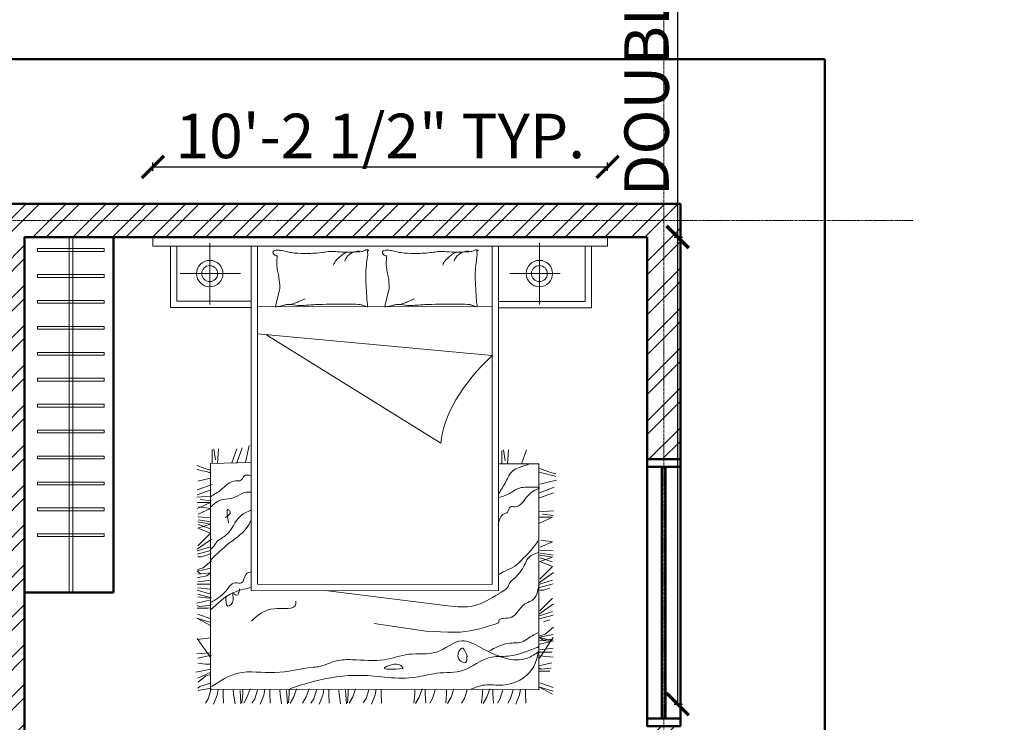
# Model space of a CAD drawing. Units: inches. Extents: x 261 to 2725, y 291 to 1454.
# Tile 15 of 35: x 777 to 1043, y 1091 to 1281. Entities that reach past the tile are written whole.
import ezdxf

# ---------------------------------------------------------------- set-up
doc = ezdxf.new("R2010")
doc.units = ezdxf.units.IN
doc.linetypes.add('CENTER', pattern=[2, 1.25, -0.25, 0.25, -0.25])
for name, color, linetype, lineweight in [('A-ANNO-DIMS', 136, 'Continuous', 18), ('A-FURN', 30, 'Continuous', 18), ('A-GRID', 251, 'CENTER', 13), ('A-WALL', 222, 'Continuous', 50), ('A-WALL-PATT', 243, 'Continuous', 13)]:
    doc.layers.add(name, color=color, linetype=linetype, lineweight=lineweight)
doc.styles.get("Standard").update_dxf_attribs({"font": 'arial.ttf'})
doc.dimstyles.new('ISO-25', dxfattribs={"dimtxt": 12, "dimasz": 6, "dimexe": 1.25, "dimexo": 0.625, "dimtad": 1, "dimdec": 0, "dimlunit": 3, "dimtxsty": 'Standard', "dimblk": 'ARCHTICK', "dimcen": 2.5, "dimadec": 0, "dimazin": 0, "dimtfac": 1, "dimtdec": 0, "dimtmove": 0, "dimatfit": 3, "dimfxl": 1, "dimfxlon": 1, "dimarcsym": 0})

# ---------------------------------------------------------------- blocks, each defined once
blk = doc.blocks.new('A$C2B723114')
for p, q in [((0, 2.9047), (2.8274, 2.9047)), ((0, 2.8487), (0, 2.9047)), ((2.8274, 2.9047), (2.8274, 2.8487)), ((2.8274, 2.8487), (0, 2.8487)), ((0.1012, 2.4649), (0.1012, 2.849)), ((0.1396, 2.5033), (0.1396, 2.849)), ((0.4243, 2.8697), (0.4243, 2.4855)), ((0.6794, 0.7051), (0.6794, 2.8509)), ((0.7187, 0.7435), (0.7187, 2.8509)), ((2.1776, 2.8509), (2.1776, 0.7454)), ((2.216, 2.8509), (2.216, 0.707)), ((2.4742, 2.8697), (2.4742, 2.4855)), ((2.6798, 2.5052), (2.6798, 2.8509)), ((2.7182, 2.4668), (2.7182, 2.8509)), ((0.6087, 2.6776), (0.295, 2.6776)), ((2.6586, 2.6776), (2.2821, 2.6776)), ((1.3789, 2.4999), (1.3598, 2.5761)), ((2.0593, 2.4999), (2.0402, 2.5761)), ((0.6794, 2.4649), (0.1012, 2.4649)), ((0.6766, 2.5033), (0.1396, 2.5033)), ((0.7191, 2.47), (2.1778, 2.4719)), ((1.3858, 2.4723), (1.3789, 2.4999)), ((2.0662, 2.4723), (2.0593, 2.4999)), ((2.2188, 2.5052), (2.6798, 2.5052)), ((2.2188, 2.4668), (2.7182, 2.4668)), ((2.1771, 2.3036), (0.718, 2.1685)), ((1.0365, 1.6233), (2.1246, 2.2989)), ((2.2287, 1.6076), (2.2523, 1.5035)), ((2.2726, 1.593), (2.3061, 1.5007)), ((0.5047, 1.5819), (0.5353, 1.4945)), ((0.6174, 1.5819), (0.6232, 1.4916)), ((0.6467, 1.5819), (0.6369, 1.5137)), ((0.6571, 1.4945), (0.6571, 1.5765)), ((2.3067, 1.5881), (2.3373, 1.5007)), ((2.4194, 1.5881), (2.4251, 1.4979)), ((2.4487, 1.5881), (2.4389, 1.5199)), ((2.4591, 1.5007), (2.4591, 1.5828)), ((0.4269, 0.0884), (0.4269, 1.4945)), ((0.4269, 1.4945), (0.6794, 1.4945)), ((2.4685, 1.4964), (2.216, 1.5022)), ((2.4685, 1.4964), (2.4685, 0.0903)), ((0.3172, 1.3923), (0.4213, 1.3687)), ((0.3318, 1.3485), (0.4241, 1.3149)), ((2.4596, 1.3659), (2.552, 1.3324)), ((2.4685, 1.4044), (2.5491, 1.3861)), ((0.3367, 1.3143), (0.4241, 1.2838)), ((2.4645, 1.3318), (2.552, 1.3012)), ((2.4645, 1.2928), (2.5548, 1.2871)), ((2.4645, 1.2635), (2.5328, 1.2733)), ((2.4699, 1.2531), (2.552, 1.2163)), ((2.552, 1.2531), (2.4699, 1.2531)), ((2.5435, 1.2276), (2.4699, 1.2163)), ((0.3367, 1.2016), (0.427, 1.1959)), ((0.3367, 1.1724), (0.405, 1.1821)), ((2.5491, 1.1654), (2.467, 1.1597)), ((2.4699, 1.2163), (2.5463, 1.1823)), ((0.4241, 1.162), (0.3421, 1.162)), ((0.3421, 1.162), (0.4241, 1.1252)), ((2.5463, 1.1455), (2.467, 1.1342)), ((2.5491, 1.1342), (2.4699, 1.1201)), ((2.4699, 1.1201), (2.5491, 1.0946)), ((2.5463, 1.1172), (2.4727, 1.0918)), ((2.5491, 1.0946), (2.4699, 1.0635)), ((2.4699, 1.0635), (2.5491, 0.9842)), ((0.4157, 1.0206), (0.3421, 1.0093)), ((0.3421, 1.0093), (0.4185, 0.9754)), ((2.4642, 1.0267), (2.552, 0.9644)), ((0.4213, 0.9584), (0.3392, 0.9527)), ((0.4185, 0.9386), (0.3392, 0.9272)), ((0.4213, 0.9272), (0.3421, 0.9131)), ((2.4642, 0.9389), (2.4869, 0.9276)), ((2.467, 0.9559), (2.552, 0.9333)), ((2.4699, 0.9785), (2.552, 0.9531)), ((2.4869, 0.9276), (2.5265, 0.9163)), ((0.3421, 0.9131), (0.4213, 0.8876)), ((0.4213, 0.8876), (0.3421, 0.8565)), ((0.4185, 0.9103), (0.3449, 0.8848)), ((2.4642, 0.8908), (2.5152, 0.8483)), ((2.5265, 0.9163), (2.5491, 0.9163)), ((0.3364, 0.8197), (0.4241, 0.7574)), ((0.3421, 0.8565), (0.4213, 0.7772)), ((2.467, 0.8455), (2.5208, 0.8342)), ((2.4699, 0.8172), (2.4925, 0.7974)), ((2.5491, 0.8087), (2.4699, 0.8172)), ((2.4925, 0.7974), (2.535, 0.7889)), ((2.5152, 0.8483), (2.5491, 0.837)), ((2.5208, 0.8342), (2.552, 0.8285)), ((2.552, 0.8285), (2.5293, 0.8087)), ((0.3392, 0.7489), (0.4241, 0.7263)), ((0.3421, 0.7716), (0.4241, 0.7461)), ((2.1776, 0.7454), (0.7187, 0.7435)), ((2.5491, 0.7606), (2.467, 0.7719)), ((2.4727, 0.7464), (2.467, 0.7408)), ((2.552, 0.7464), (2.4727, 0.7464)), ((2.535, 0.7889), (2.552, 0.7861)), ((0.359, 0.7206), (0.3987, 0.7093)), ((0.3987, 0.7093), (0.4213, 0.7093)), ((2.216, 0.707), (0.6794, 0.7051)), ((0.9938, 0.6115), (1.7555, 0.7064)), ((2.5491, 0.6842), (2.4642, 0.6615)), ((2.467, 0.7153), (2.5491, 0.7238)), ((2.552, 0.7096), (2.467, 0.6842)), ((0.3364, 0.6233), (0.4241, 0.561)), ((0.3421, 0.6601), (0.4213, 0.5808)), ((2.4642, 0.6191), (2.4784, 0.6134)), ((2.5491, 0.6672), (2.4755, 0.6587)), ((2.4755, 0.6474), (2.5548, 0.6276)), ((2.4784, 0.6134), (2.5406, 0.6077)), ((2.5406, 0.6077), (2.552, 0.6134)), ((0.3392, 0.5525), (0.4241, 0.5299)), ((0.3421, 0.5752), (0.4241, 0.5497)), ((2.467, 0.5993), (2.4869, 0.5964)), ((2.467, 0.5313), (2.5491, 0.5596)), ((2.4869, 0.5964), (2.552, 0.5964)), ((0.359, 0.5242), (0.3987, 0.5129)), ((1.4523, 0.5021), (1.1305, 0.4537)), ((2.467, 0.5087), (2.5548, 0.5342)), ((2.5548, 0.5342), (2.4699, 0.4889)), ((0.3364, 0.4785), (0.3874, 0.436)), ((0.3392, 0.4332), (0.393, 0.4219)), ((0.3874, 0.436), (0.4213, 0.4247)), ((1.1305, 0.4537), (0.9938, 0.448)), ((0.4213, 0.415), (0.3364, 0.3923)), ((0.4241, 0.2868), (0.3392, 0.415)), ((0.3421, 0.4049), (0.3647, 0.3851)), ((0.4213, 0.3964), (0.3421, 0.4049)), ((0.4213, 0.398), (0.3477, 0.3895)), ((0.3647, 0.3851), (0.4072, 0.3766)), ((0.393, 0.4219), (0.4241, 0.4162)), ((0.4241, 0.4162), (0.4015, 0.3964)), ((0.4072, 0.3766), (0.4241, 0.3738)), ((2.467, 0.4133), (2.552, 0.4019)), ((2.467, 0.2879), (2.552, 0.4076)), ((0.4213, 0.3377), (0.3392, 0.3491)), ((0.4241, 0.3236), (0.3449, 0.3236)), ((2.467, 0.319), (2.5548, 0.3134)), ((0.3392, 0.2925), (0.4213, 0.3009)), ((0.3477, 0.2571), (0.427, 0.2373)), ((2.4642, 0.3049), (2.5491, 0.2851)), ((2.4699, 0.2491), (2.501, 0.2491)), ((2.501, 0.2491), (2.5491, 0.2547)), ((0.3506, 0.2231), (0.4128, 0.2175)), ((0.359, 0.2061), (0.4241, 0.2061)), ((0.4128, 0.2175), (0.4241, 0.2231)), ((2.467, 0.2179), (2.5605, 0.1981)), ((2.467, 0.1981), (2.5491, 0.1613)), ((2.467, 0.184), (2.4982, 0.1755)), ((0.3392, 0.1042), (0.4213, 0.1325)), ((2.4699, 0.1302), (2.535, 0.1104)), ((2.4982, 0.1755), (2.5463, 0.1359)), ((0.3392, 0.0815), (0.427, 0.107)), ((0.427, 0.107), (0.3421, 0.0617)), ((2.4685, 0.0903), (0.4269, 0.0884)), ((0.5106, 0.0657), (0.5077, 0.0063)), ((0.5106, 0.094), (0.5106, 0.0657)), ((0.5417, 0.094), (0.5474, 0.0572)), ((0.587, 0.0884), (0.604, 0.0346)), ((0.6512, 0.0884), (0.6682, 0.0346)), ((0.713, 0.0657), (0.7101, 0.0063)), ((0.713, 0.094), (0.713, 0.0657)), ((0.7334, 0.0943), (0.7503, 0.0434)), ((0.7786, 0.0915), (0.7786, 0.0632)), ((0.7786, 0.0632), (0.7843, 0.0066)), ((0.8739, 0.0884), (0.8908, 0.0346)), ((0.956, 0.0943), (0.973, 0.0434)), ((1.0013, 0.0915), (1.0013, 0.0632)), ((1.0013, 0.0632), (1.007, 0.0066)), ((1.072, 0.0884), (1.089, 0.0346)), ((1.1338, 0.0657), (1.131, 0.0063)), ((1.1338, 0.094), (1.1338, 0.0657)), ((1.1542, 0.0943), (1.1712, 0.0434)), ((1.1995, 0.0915), (1.1995, 0.0632)), ((1.1995, 0.0632), (1.2052, 0.0066)), ((1.4088, 0.0657), (1.406, 0.0063)), ((1.4088, 0.094), (1.4088, 0.0657)), ((1.44, 0.094), (1.4456, 0.0572)), ((1.4853, 0.0884), (1.5023, 0.0346)), ((1.5674, 0.0962), (1.5844, 0.0453)), ((1.6127, 0.0934), (1.6127, 0.0651)), ((1.6127, 0.0651), (1.6184, 0.0085)), ((1.6297, 0.0849), (1.624, 0.0028)), ((1.6693, 0.0623), (1.6608, 0.0028)), ((1.6721, 0.0877), (1.6693, 0.0623)), ((1.7344, 0.0651), (1.7316, 0.0057)), ((1.7344, 0.0934), (1.7344, 0.0651)), ((1.7655, 0.0934), (1.7712, 0.0566)), ((1.8108, 0.0877), (1.8278, 0.034)), ((1.8568, 0.0962), (1.8738, 0.0453)), ((1.9342, 0.0962), (1.9512, 0.0453)), ((1.9795, 0.0934), (1.9795, 0.0651)), ((1.9795, 0.0651), (1.9852, 0.0085)), ((1.9965, 0.0849), (1.9908, 0.0028)), ((2.0361, 0.0623), (2.0276, 0.0028)), ((2.039, 0.0877), (2.0361, 0.0623)), ((2.1012, 0.0651), (2.0984, 0.0057)), ((2.1012, 0.0934), (2.1012, 0.0651)), ((2.1324, 0.0934), (2.138, 0.0566)), ((2.1777, 0.0877), (2.1946, 0.034)), ((2.2236, 0.0962), (2.2406, 0.0453)), ((2.2689, 0.0934), (2.2689, 0.0651)), ((2.2689, 0.0651), (2.2746, 0.0085)), ((2.2859, 0.0849), (2.2802, 0.0028)), ((2.3255, 0.0623), (2.317, 0.0028)), ((2.3284, 0.0877), (2.3255, 0.0623)), ((2.3906, 0.0651), (2.3878, 0.0057)), ((2.3906, 0.0934), (2.3906, 0.0651)), ((2.4218, 0.0934), (2.4274, 0.0566)), ((2.4642, 0.0991), (2.5378, 0.0877)), ((2.467, 0.0877), (2.484, 0.034)), ((2.535, 0.1104), (2.5491, 0.0991)), ((2.5378, 0.0877), (2.5463, 0.0821)), ((0.5474, 0.0572), (0.57, 0.0006)), ((0.604, 0.0346), (0.621, 0.0063)), ((0.6682, 0.0346), (0.6851, 0.0063)), ((0.7503, 0.0434), (0.773, 0.0037)), ((0.8908, 0.0346), (0.9078, 0.0063)), ((0.973, 0.0434), (0.9957, 0.0037)), ((1.089, 0.0346), (1.106, 0.0063)), ((1.1712, 0.0434), (1.1939, 0.0037)), ((1.4456, 0.0572), (1.4683, 0.0006)), ((1.5023, 0.0346), (1.5192, 0.0082)), ((1.5844, 0.0453), (1.607, 0.0057)), ((1.7712, 0.0566), (1.7938, 0)), ((1.8278, 0.034), (1.8448, 0.0057)), ((1.8738, 0.0453), (1.8964, 0.0057)), ((1.9512, 0.0453), (1.9739, 0.0057)), ((2.138, 0.0566), (2.1607, 0)), ((2.1946, 0.034), (2.2116, 0.0057)), ((2.2406, 0.0453), (2.2632, 0.0057)), ((2.4274, 0.0566), (2.4501, 0)), ((2.484, 0.034), (2.501, 0.0057))]:
    blk.add_line(p, q)
for centre, radius in [((0.4243, 2.6776), 0.0821), ((2.4742, 2.6776), 0.0821), ((0.4243, 2.6776), 0.0493), ((2.4742, 2.6776), 0.0493)]:
    blk.add_circle(centre, radius)
for centre, radius, start, end in [((0.8078, 2.821), 0.00214, 160.43603, 281.89306), ((0.8088, 2.8207), 0.00315, 111.7883, 160.43603), ((0.8162, 2.8021), 0.0232, 94.30254, 111.7883), ((0.8091, 2.8151), 0.00394, 21.9904, 101.89306), ((0.7994, 2.8112), 0.0144, 338.57902, 21.9904), ((0.8165, 2.7987), 0.0266, 59.34875, 94.30254), ((0.8554, 2.8643), 0.0497, 239.34875, 264.74081), ((0.8679, 2.7254), 0.0915, 74.06476, 94.21588), ((1.3941, 2.5438), 0.281, 98.43719, 105.74398), ((1.3747, 2.6748), 0.1486, 90, 98.43719), ((1.3747, 2.74), 0.0833, 78.72762, 90), ((1.3886, 2.8099), 0.0121, 333.41948, 78.72762), ((1.4882, 2.821), 0.00214, 160.43603, 281.89306), ((1.4892, 2.8207), 0.00315, 111.7883, 160.43603), ((1.4966, 2.8021), 0.0232, 94.30254, 111.7883), ((1.4895, 2.8151), 0.00394, 21.9904, 101.89306), ((1.4798, 2.8112), 0.0144, 338.57902, 21.9904), ((1.4969, 2.7987), 0.0266, 59.34875, 94.30254), ((1.5358, 2.8643), 0.0497, 239.34875, 264.74081), ((1.5483, 2.7254), 0.0915, 74.06476, 94.21588), ((2.0745, 2.5438), 0.281, 98.43719, 105.74398), ((2.0551, 2.6748), 0.1486, 90, 98.43719), ((2.0551, 2.74), 0.0833, 78.72762, 90), ((2.069, 2.8099), 0.0121, 333.41948, 78.72762), ((0.8409, 2.7949), 0.0302, 158.57902, 188.13348), ((1.0356, 2.8227), 0.2268, 188.13348, 192.10946), ((0.635, 2.7368), 0.1829, 7.6809, 12.10946), ((-0.0181, 2.6487), 0.8418, 3.36875, 7.6809), ((0.9202, 3.5684), 0.7568, 264.74081, 268.09211), ((0.8679, 2.7254), 0.0915, 53.91364, 74.06476), ((0.9409, 4.189), 1.3777, 268.09211, 270.57574), ((0.8679, 2.7254), 0.0915, 36.17665, 53.91364), ((0.86, 2.6097), 0.2158, 62.76041, 69.13972), ((0.8679, 2.7254), 0.0915, 18.43965, 36.17665), ((0.9466, 3.6164), 0.8051, 270.57574, 274.80185), ((0.9263, 2.7386), 0.0708, 51.61143, 62.76041), ((0.7461, 2.511), 0.3611, 46.18849, 51.61143), ((0.8523, 2.6218), 0.2076, 39.03494, 46.18849), ((1.0364, 2.548), 0.2671, 87.46141, 94.80185), ((1.042, 2.6745), 0.1405, 79.81012, 87.46141), ((1.1532, 3.2931), 0.488, 259.81012, 263.9133), ((1.204, 3.7695), 0.9671, 263.9133, 270), ((1.204, 3.4318), 0.6294, 270, 277.54685), ((1.2573, 3.0292), 0.2233, 277.54685, 285.74398), ((1.3713, 2.8186), 0.0315, 274.40021, 333.41948), ((0.923, 2.7382), 0.4535, 0, 6.23236), ((1.5213, 2.7949), 0.0302, 158.57902, 188.13348), ((1.716, 2.8227), 0.2268, 188.13348, 192.10946), ((1.3154, 2.7368), 0.1829, 7.6809, 12.10946), ((0.6623, 2.6487), 0.8418, 3.36875, 7.6809), ((1.6006, 3.5684), 0.7568, 264.74081, 268.09211), ((1.5483, 2.7254), 0.0915, 53.91364, 74.06476), ((1.6213, 4.189), 1.3777, 268.09211, 270.57574), ((1.5483, 2.7254), 0.0915, 36.17665, 53.91364), ((1.5404, 2.6097), 0.2158, 62.76041, 69.13972), ((1.5483, 2.7254), 0.0915, 18.43965, 36.17665), ((1.627, 3.6164), 0.8051, 270.57574, 274.80185), ((1.6067, 2.7386), 0.0708, 51.61143, 62.76041), ((1.4265, 2.511), 0.3611, 46.18849, 51.61143), ((1.5327, 2.6218), 0.2076, 39.03494, 46.18849), ((1.7168, 2.548), 0.2671, 87.46141, 94.80185), ((1.7224, 2.6745), 0.1405, 79.81012, 87.46141), ((1.8336, 3.2931), 0.488, 259.81012, 263.9133), ((1.8844, 3.7695), 0.9671, 263.9133, 270), ((1.8844, 3.4318), 0.6294, 270, 277.54685), ((1.9377, 3.0292), 0.2233, 277.54685, 285.74398), ((2.0517, 2.8186), 0.0315, 274.40021, 333.41948), ((1.6034, 2.7382), 0.4535, 0, 6.23236), ((0.1976, 2.6614), 0.6258, 358.36691, 3.36875), ((0.9783, 2.7239), 0.0455, 28.31676, 39.03494), ((0.8558, 2.6579), 0.1846, 23.00277, 28.31676), ((0.5722, 2.8434), 0.8132, 347.80162, 350.31563), ((1.1884, 2.7382), 0.1881, 350.31563, 0), ((0.878, 2.6614), 0.6258, 358.36691, 3.36875), ((1.6587, 2.7239), 0.0455, 28.31676, 39.03494), ((1.5362, 2.6579), 0.1846, 23.00277, 28.31676), ((1.2526, 2.8434), 0.8132, 347.80162, 350.31563), ((1.8688, 2.7382), 0.1881, 350.31563, 0), ((-0.4351, 2.6794), 1.2587, 356.94504, 358.36691), ((1.9648, 2.5659), 0.6074, 171.99495, 177.33512), ((1.6528, 2.6098), 0.2924, 167.80162, 171.99495), ((0.2453, 2.6794), 1.2587, 356.94504, 358.36691), ((2.6452, 2.5659), 0.6074, 171.99495, 177.33512), ((2.3332, 2.6098), 0.2924, 167.80162, 171.99495), ((-11.7321, 3.2823), 12.5718, 356.49514, 356.94504), ((1.4204, 2.5912), 0.0624, 177.33512, 194.04519), ((-11.0517, 3.2823), 12.5718, 356.49514, 356.94504), ((2.1008, 2.5912), 0.0624, 177.33512, 194.04519), ((0.5206, 2.5319), 0.2961, 350.00164, 356.49514), ((1.4917, 3.1364), 0.681, 244.68893, 246.51559), ((1.4917, 3.1364), 0.681, 246.51559, 248.34226), ((1.201, 2.5319), 0.2961, 350.00164, 356.49514), ((2.1721, 3.1364), 0.681, 244.68893, 246.51559), ((2.1721, 3.1364), 0.681, 246.51559, 248.34226), ((0.8298, 2.4774), 0.0178, 170.00164, 196.69777), ((0.8139, 2.4726), 0.00122, 196.69777, 277.12039), ((0.8041, 2.5514), 0.0807, 277.12039, 286.22115), ((0.8068, 2.5419), 0.0707, 286.22115, 297.28412), ((0.8584, 2.4419), 0.0418, 102.86904, 117.28412), ((0.879, 2.3515), 0.1345, 93.57397, 102.86904), ((0.9376, 1.4146), 1.0732, 90.28654, 93.57397), ((0.9586, -2.7845), 5.2724, 89.02962, 90.28654), ((0.9954, -0.6123), 3.0999, 87.39037, 89.02962), ((1.0854, 1.364), 1.1216, 85.38242, 87.39037), ((1.28, 3.7729), 1.2952, 265.38242, 267.25094), ((1.228, 2.691), 0.2121, 267.25094, 281.55856), ((1.4917, 3.1364), 0.681, 248.34226, 250.57202), ((1.4917, 3.1364), 0.681, 250.57202, 252.80178), ((1.2975, 2.3514), 0.1345, 83.56595, 101.55856), ((1.3002, 2.3754), 0.1104, 72.61359, 83.56595), ((1.3965, 2.6828), 0.2118, 252.61359, 260.5159), ((1.4027, 2.7202), 0.2496, 260.5159, 265.91706), ((1.385, 2.4721), 0.000845, 265.91706, 14.04494), ((1.5102, 2.4774), 0.0178, 170.00164, 196.69777), ((1.4943, 2.4726), 0.00122, 196.69777, 277.12039), ((1.4845, 2.5514), 0.0807, 277.12039, 286.22115), ((1.4872, 2.5419), 0.0707, 286.22115, 297.28412), ((1.5388, 2.4419), 0.0418, 102.86904, 117.28412), ((1.5594, 2.3515), 0.1345, 93.57397, 102.86904), ((1.618, 1.4146), 1.0732, 90.28654, 93.57397), ((1.639, -2.7845), 5.2724, 89.02962, 90.28654), ((1.6758, -0.6123), 3.0999, 87.39037, 89.02962), ((1.7658, 1.364), 1.1216, 85.38242, 87.39037), ((1.9604, 3.7729), 1.2952, 265.38242, 267.25094), ((1.9084, 2.691), 0.2121, 267.25094, 281.55856), ((2.1721, 3.1364), 0.681, 248.34226, 250.57202), ((2.1721, 3.1364), 0.681, 250.57202, 252.80178), ((1.9779, 2.3514), 0.1345, 83.56595, 101.55856), ((1.9806, 2.3754), 0.1104, 72.61359, 83.56595), ((2.0769, 2.6828), 0.2118, 252.61359, 260.5159), ((2.0831, 2.7202), 0.2496, 260.5159, 265.91706), ((2.0654, 2.4721), 0.000845, 265.91706, 14.04494)]:
    blk.add_arc(centre, radius, start, end)
blk.add_ellipse((0.4962, 1.9132), major_axis=(0.4887, -0.4605), ratio=0.503305, start_param=0.491272, end_param=1.591113)
for points, knots in [([(0.6768, 1.3104), (0.6615, 1.3339), (0.6315, 1.3797), (0.604, 1.4501), (0.5417, 1.4748), (0.5064, 1.4871), (0.4848, 1.4945)], [0, 0, 0, 0, 110.980521, 216.571322, 273.316778, 363.252298, 363.252298, 363.252298, 363.252298]), ([(2.5548, 1.4853), (2.5314, 1.4757), (2.5031, 1.4641), (2.4737, 1.4555), (2.4685, 1.454)], [0, 0, 0, 0, 98.452083, 119.481049, 119.481049, 119.481049, 119.481049]), ([(0.427, 1.4678), (0.4036, 1.4582), (0.3693, 1.4441), (0.3335, 1.4344), (0.3221, 1.4313)], [0, 0, 0, 0, 98.452083, 144.639601, 144.639601, 144.639601, 144.639601]), ([(0.4241, 1.4423), (0.4031, 1.437), (0.3691, 1.4284), (0.3351, 1.4199), (0.3221, 1.4167)], [0, 0, 0, 0, 84.638756, 136.955563, 136.955563, 136.955563, 136.955563]), ([(2.2145, 1.4211), (2.233, 1.4246), (2.2636, 1.4303), (2.2761, 1.3837), (2.3429, 1.3967), (2.3949, 1.3342), (2.4474, 1.3031), (2.4698, 1.2898)], [0, 0, 0, 0, 61.886907, 102.717887, 145.699352, 284.082577, 386.765171, 386.765171, 386.765171, 386.765171]), ([(2.552, 1.4598), (2.5309, 1.4545), (2.5031, 1.4475), (2.4753, 1.4406), (2.4685, 1.4389)], [0, 0, 0, 0, 84.638756, 111.94623, 111.94623, 111.94623, 111.94623]), ([(0.6768, 1.286), (0.6567, 1.2911), (0.6145, 1.3017), (0.5543, 1.3533), (0.4816, 1.349), (0.4362, 1.3493), (0.4233, 1.3493)], [0, 0, 0, 0, 80.250278, 168.388677, 295.908361, 346.663112, 346.663112, 346.663112, 346.663112]), ([(0.4233, 1.3445), (0.4367, 1.3385), (0.464, 1.3264), (0.5129, 1.2848), (0.5456, 1.2161), (0.6131, 1.2349), (0.6142, 1.1913), (0.6642, 1.1806), (0.674, 1.144), (0.6817, 1.1154)], [0, 0, 0, 0, 56.745495, 115.23739, 254.956954, 286.678662, 337.828324, 366.201072, 468.500395, 468.500395, 468.500395, 468.500395]), ([(2.2145, 1.319), (2.2295, 1.319), (2.2678, 1.3192), (2.3288, 1.2705), (2.4143, 1.279), (2.4535, 1.2403), (2.4662, 1.2278)], [0, 0, 0, 0, 57.155505, 146.33427, 287.936209, 355.396728, 355.396728, 355.396728, 355.396728]), ([(2.3573, 1.127), (2.3656, 1.1759), (2.3758, 1.2352), (2.3371, 1.1853), (2.3602, 1.1713), (2.3768, 1.1612)], [0, 0, 0, 0, 107.853607, 130.728419, 189.220329, 189.220329, 189.220329, 189.220329]), ([(2.2182, 1.2059), (2.2419, 1.1958), (2.3116, 1.1659), (2.342, 1.0552), (2.4266, 1.0223), (2.4474, 0.9811), (2.462, 0.9684), (2.4698, 0.9616)], [0, 0, 0, 0, 97.73655, 287.59661, 389.176293, 423.403759, 463.679181, 463.679181, 463.679181, 463.679181]), ([(2.2145, 1.1476), (2.2246, 1.1286), (2.2575, 1.0666), (2.3612, 1.0009), (2.431, 0.9336), (2.4662, 0.8996)], [0, 0, 0, 0, 83.02987, 271.460712, 463.033803, 463.033803, 463.033803, 463.033803]), ([(0.6817, 0.8034), (0.6673, 0.8119), (0.6341, 0.8315), (0.5785, 0.8518), (0.5349, 0.8973), (0.4828, 0.9461), (0.4518, 0.9879), (0.4331, 1.013)], [0, 0, 0, 0, 65.318952, 150.437229, 226.833166, 307.58338, 429.454095, 429.454095, 429.454095, 429.454095]), ([(0.4282, 0.9448), (0.4547, 0.9353), (0.496, 0.9206), (0.5223, 0.8436), (0.5628, 0.7946), (0.6113, 0.7575), (0.6214, 0.7173), (0.6539, 0.7022), (0.672, 0.6897), (0.6768, 0.6864)], [0, 0, 0, 0, 102.299436, 159.044876, 303.717955, 348.579152, 391.138254, 454.581655, 477.456496, 477.456496, 477.456496, 477.456496]), ([(2.2145, 0.823), (2.227, 0.8201), (2.261, 0.8121), (2.261, 0.7401), (2.3352, 0.7659), (2.379, 0.6836), (2.4336, 0.6521), (2.4662, 0.6334)], [0, 0, 0, 0, 46.747668, 127.438174, 179.649794, 280.561838, 429.605131, 429.605131, 429.605131, 429.605131]), ([(0.4282, 0.74), (0.4347, 0.7029), (0.444, 0.6496), (0.5194, 0.6274), (0.555, 0.5807), (0.5975, 0.5243), (0.6789, 0.5415), (0.677, 0.5095), (0.6768, 0.5061)], [0, 0, 0, 0, 130.791737, 187.537266, 286.231946, 353.673191, 460.023761, 472.712403, 472.712403, 472.712403, 472.712403]), ([(0.6768, 0.6864), (0.7275, 0.655), (0.8251, 0.5944), (0.9391, 0.606), (0.9938, 0.6115)], [0, 0, 0, 0, 225.995823, 434.686543, 434.686543, 434.686543, 434.686543]), ([(2.2218, 0.7246), (2.2595, 0.716), (2.3548, 0.6945), (2.4265, 0.6268), (2.4698, 0.586)], [0, 0, 0, 0, 148.665024, 375.555892, 375.555892, 375.555892, 375.555892]), ([(2.3719, 0.6737), (2.3738, 0.6431), (2.3772, 0.5878), (2.3146, 0.6382), (2.3401, 0.7015), (2.2971, 0.6649), (2.2923, 0.6965), (2.289, 0.7176)], [0, 0, 0, 0, 83.446591, 150.887818, 201.642461, 230.015204, 286.760644, 286.760644, 286.760644, 286.760644]), ([(2.2145, 0.5167), (2.1764, 0.5522), (2.1051, 0.6184), (1.9357, 0.5803), (1.9385, 0.6342), (1.9388, 0.6395)], [0, 0, 0, 0, 208.073343, 389.01094, 409.01094, 409.01094, 409.01094, 409.01094]), ([(0.6768, 0.5061), (0.7554, 0.4794), (0.8591, 0.4442), (0.9675, 0.4473), (0.9938, 0.448)], [0, 0, 0, 0, 319.374611, 421.61723, 421.61723, 421.61723, 421.61723]), ([(0.4331, 0.4427), (0.4498, 0.4356), (0.4827, 0.4216), (0.5314, 0.3759), (0.632, 0.3884), (0.6996, 0.3513), (0.7423, 0.3278)], [0, 0, 0, 0, 70.931849, 139.556414, 248.154027, 434.709995, 434.709995, 434.709995, 434.709995]), ([(2.4625, 0.1088), (2.4095, 0.1438), (2.2904, 0.2226), (2.0623, 0.1771), (1.9006, 0.2246), (1.7699, 0.2337), (1.6941, 0.2766), (1.5528, 0.2786), (1.4005, 0.2587), (1.2324, 0.3267), (1.059, 0.2939), (0.9218, 0.426), (0.7359, 0.3204), (0.5586, 0.2391), (0.4502, 0.3116), (0.427, 0.3272)], [0, 0, 0, 0, 239.874704, 538.942419, 850.40885, 893.390315, 1047.998294, 1176.505142, 1437.500972, 1637.333004, 1864.324391, 2089.058767, 2248.736533, 2637.953392, 2744.252142, 2744.252142, 2744.252142, 2744.252142]), ([(1.9771, 0.0962), (1.9286, 0.1117), (1.7864, 0.157), (1.5223, 0.1992), (1.2611, 0.141), (1.0527, 0.2023), (0.8859, 0.1885), (0.76, 0.3042), (0.6211, 0.292), (0.5187, 0.3203), (0.4572, 0.3456), (0.4282, 0.3575)], [0, 0, 0, 0, 198.710624, 582.73994, 1031.873213, 1206.082894, 1423.278209, 1655.952104, 1808.744089, 1945.69963, 2068.229211, 2068.229211, 2068.229211, 2068.229211]), ([(0.8474, 0.0943), (0.82, 0.1047), (0.757, 0.1287), (0.6201, 0.1029), (0.4623, 0.1837), (0.4372, 0.2936), (0.4282, 0.3331)], [0, 0, 0, 0, 112.422038, 258.341957, 533.791494, 688.286079, 688.286079, 688.286079, 688.286079]), ([(0.8718, 0.2941), (0.8821, 0.3221), (0.9041, 0.3814), (0.9523, 0.2773), (0.8733, 0.2454), (0.8757, 0.2798), (0.8766, 0.2941)], [0, 0, 0, 0, 82.720021, 175.094899, 237.579423, 282.440623, 282.440623, 282.440623, 282.440623]), ([(1.2715, 0.221), (1.3344, 0.2172), (1.4529, 0.21), (1.2971, 0.2665), (1.2756, 0.2284), (1.2715, 0.221)], [0, 0, 0, 0, 150.888188, 283.977876, 315.699589, 315.699589, 315.699589, 315.699589])]:
    blk.add_open_spline(points, degree=3, knots=knots)
blk = doc.blocks.new('_ArchTick')
at = {"color": 0, "linetype": 'ByBlock', "const_width": 0.15}
blk.add_lwpolyline([(-0.5, -0.5), (0.5, 0.5)], dxfattribs=at)
blk = doc.blocks.new('*D41')
at = {"layer": 'A-ANNO-DIMS', "color": 0, "lineweight": -2, "ltscale": 0.07, "transparency": 16777216}
for p, q in [((954.74, 1222.47), (954.74, 1424.31)), ((953.74, 1222.47), (955.99, 1222.47)), ((954.74, 1096.37), (954.74, 1222.47)), ((953.74, 1096.37), (955.99, 1096.37))]:
    blk.add_line(p, q, dxfattribs=at)
at = {"layer": 'Defpoints', "color": 0, "ltscale": 0.07, "transparency": 16777216}
for p in [(935.82, 1222.47), (954.74, 1222.47), (935.82, 1096.37)]:
    blk.add_point(p, dxfattribs=at)
at = {"layer": 'A-ANNO-DIMS', "color": 0, "lineweight": -2, "ltscale": 0.07, "transparency": 16777216, "xscale": 6, "yscale": 6, "zscale": 6}
for p, rotation in [((954.74, 1222.47), 90), ((954.74, 1096.37), 270)]:
    blk.add_blockref('_ArchTick', p, dxfattribs=dict(at, rotation=rotation))
at = {"layer": 'A-ANNO-DIMS', "color": 0, "ltscale": 0.07, "transparency": 16777216, "insert": (947.9, 1326.39), "char_height": 12, "attachment_point": 5, "rotation": 90}
blk.add_mtext('DOUBLE BED 10\'-6" TYP.', dxfattribs=at)
blk = doc.blocks.new('*D42')
at = {"layer": 'A-ANNO-DIMS', "color": 0, "lineweight": -2, "ltscale": 0.07, "transparency": 16777216}
for p, q in [((813.08, 1240.38), (813.08, 1242.63)), ((935.82, 1241.38), (813.08, 1241.38)), ((935.82, 1240.38), (935.82, 1242.63))]:
    blk.add_line(p, q, dxfattribs=at)
at = {"layer": 'Defpoints', "color": 0, "ltscale": 0.07, "transparency": 16777216}
for p in [(813.08, 1241.38), (813.08, 1222.47), (935.82, 1222.47)]:
    blk.add_point(p, dxfattribs=at)
at = {"layer": 'A-ANNO-DIMS', "color": 0, "lineweight": -2, "ltscale": 0.07, "transparency": 16777216, "xscale": 6, "yscale": 6, "zscale": 6, "rotation": 180}
blk.add_blockref('_ArchTick', (813.08, 1241.38), dxfattribs=at)
at = {"layer": 'A-ANNO-DIMS', "color": 0, "lineweight": -2, "ltscale": 0.07, "transparency": 16777216, "xscale": 6, "yscale": 6, "zscale": 6}
blk.add_blockref('_ArchTick', (935.82, 1241.38), dxfattribs=at)
at = {"layer": 'A-ANNO-DIMS', "color": 0, "ltscale": 0.07, "transparency": 16777216, "insert": (874.45, 1248.21), "char_height": 12, "attachment_point": 5}
blk.add_mtext('10\'-2 1/2" TYP.', dxfattribs=at)
blk = doc.blocks.new('*D76')
at = {"layer": 'A-ANNO-DIMS', "color": 0, "lineweight": -2, "ltscale": 0.07, "transparency": 16777216}
for p, q in [((772.45, 1437.76), (772.45, 1440.01)), ((772.45, 1438.76), (946.45, 1438.76)), ((946.45, 1437.76), (946.45, 1440.01))]:
    blk.add_line(p, q, dxfattribs=at)
at = {"layer": 'Defpoints', "color": 0, "ltscale": 0.07, "transparency": 16777216}
for p in [(946.45, 1438.76), (772.45, 1222.47), (946.45, 1222.47)]:
    blk.add_point(p, dxfattribs=at)
at = {"layer": 'A-ANNO-DIMS', "color": 0, "lineweight": -2, "ltscale": 0.07, "transparency": 16777216, "xscale": 6, "yscale": 6, "zscale": 6, "rotation": 180}
blk.add_blockref('_ArchTick', (772.45, 1438.76), dxfattribs=at)
at = {"layer": 'A-ANNO-DIMS', "color": 0, "lineweight": -2, "ltscale": 0.07, "transparency": 16777216, "xscale": 6, "yscale": 6, "zscale": 6}
blk.add_blockref('_ArchTick', (946.45, 1438.76), dxfattribs=at)
at = {"layer": 'A-ANNO-DIMS', "color": 0, "ltscale": 0.07, "transparency": 16777216, "insert": (859.45, 1445.51), "char_height": 12, "attachment_point": 5}
blk.add_mtext('14\'-6"', dxfattribs=at)
blk = doc.blocks.new('*D85')
at = {"layer": 'A-ANNO-DIMS', "color": 0, "lineweight": -2, "ltscale": 0.07, "transparency": 16777216}
for p, q in [((2600.96, 1222.47), (2603.21, 1222.47)), ((2601.96, 1024.47), (2601.96, 1222.47)), ((2600.96, 1024.47), (2603.21, 1024.47))]:
    blk.add_line(p, q, dxfattribs=at)
at = {"layer": 'Defpoints', "color": 0, "ltscale": 0.07, "transparency": 16777216}
for p in [(946.45, 1222.47), (2601.96, 1222.47), (946.45, 1024.47)]:
    blk.add_point(p, dxfattribs=at)
at = {"layer": 'A-ANNO-DIMS', "color": 0, "lineweight": -2, "ltscale": 0.07, "transparency": 16777216, "xscale": 6, "yscale": 6, "zscale": 6}
for p, rotation in [((2601.96, 1222.47), 90), ((2601.96, 1024.47), 270)]:
    blk.add_blockref('_ArchTick', p, dxfattribs=dict(at, rotation=rotation))
at = {"layer": 'A-ANNO-DIMS', "color": 0, "ltscale": 0.07, "transparency": 16777216, "insert": (2595.21, 1123.47), "char_height": 12, "attachment_point": 5, "rotation": 90}
blk.add_mtext('16\'-6"', dxfattribs=at)
blk = doc.blocks.new('*D103')
at = {"layer": 'A-ANNO-DIMS', "color": 0, "lineweight": -2, "ltscale": 0.07, "transparency": 16777216}
for p, q in [((287.06, 1231.47), (284.81, 1231.47)), ((286.06, 439.47), (286.06, 1231.47)), ((287.06, 439.47), (284.81, 439.47))]:
    blk.add_line(p, q, dxfattribs=at)
at = {"layer": 'Defpoints', "color": 0, "ltscale": 0.07, "transparency": 16777216}
for p in [(286.06, 1231.47), (1243.08, 1231.47), (1243.08, 439.47)]:
    blk.add_point(p, dxfattribs=at)
at = {"layer": 'A-ANNO-DIMS', "color": 0, "lineweight": -2, "ltscale": 0.07, "transparency": 16777216, "xscale": 6, "yscale": 6, "zscale": 6}
for p, rotation in [((286.06, 1231.47), 90), ((286.06, 439.47), 270)]:
    blk.add_blockref('_ArchTick', p, dxfattribs=dict(at, rotation=rotation))
at = {"layer": 'A-ANNO-DIMS', "color": 0, "ltscale": 0.07, "transparency": 16777216, "insert": (279.3, 835.47), "char_height": 12, "attachment_point": 5, "rotation": 90}
blk.add_mtext('66\'-0"', dxfattribs=at)
blk = doc.blocks.new('*D110')
at = {"layer": 'A-ANNO-DIMS', "color": 0, "lineweight": -2, "ltscale": 0.07, "transparency": 16777216}
for p, q in [((287.06, 1222.47), (284.81, 1222.47)), ((286.06, 964.47), (286.06, 1222.47)), ((287.06, 964.47), (284.81, 964.47))]:
    blk.add_line(p, q, dxfattribs=at)
at = {"layer": 'Defpoints', "color": 0, "ltscale": 0.07, "transparency": 16777216}
for p in [(286.06, 1222.47), (1252.08, 1222.47), (1252.08, 964.47)]:
    blk.add_point(p, dxfattribs=at)
at = {"layer": 'A-ANNO-DIMS', "color": 0, "lineweight": -2, "ltscale": 0.07, "transparency": 16777216, "xscale": 6, "yscale": 6, "zscale": 6}
for p, rotation in [((286.06, 1222.47), 90), ((286.06, 964.47), 270)]:
    blk.add_blockref('_ArchTick', p, dxfattribs=dict(at, rotation=rotation))
at = {"layer": 'A-ANNO-DIMS', "color": 0, "ltscale": 0.07, "transparency": 16777216, "insert": (279.3, 1093.47), "char_height": 12, "attachment_point": 5, "rotation": 90}
blk.add_mtext('21\'-6"', dxfattribs=at)
blk = doc.blocks.new('*D118')
at = {"layer": 'A-ANNO-DIMS', "color": 0, "lineweight": -2, "ltscale": 0.07, "transparency": 16777216}
for p, q in [((287.06, 1222.47), (284.81, 1222.47)), ((286.06, 1222.47), (286.06, 1195.47)), ((287.06, 1195.47), (284.81, 1195.47)), ((286.06, 1195.47), (286.06, 1156.11))]:
    blk.add_line(p, q, dxfattribs=at)
at = {"layer": 'Defpoints', "color": 0, "ltscale": 0.07, "transparency": 16777216}
for p in [(1252.08, 1222.47), (286.06, 1195.47), (1252.08, 1195.47)]:
    blk.add_point(p, dxfattribs=at)
at = {"layer": 'A-ANNO-DIMS', "color": 0, "lineweight": -2, "ltscale": 0.07, "transparency": 16777216, "xscale": 6, "yscale": 6, "zscale": 6}
for p, rotation in [((286.06, 1222.47), 90), ((286.06, 1195.47), 270)]:
    blk.add_blockref('_ArchTick', p, dxfattribs=dict(at, rotation=rotation))
at = {"layer": 'A-ANNO-DIMS', "color": 0, "ltscale": 0.07, "transparency": 16777216, "insert": (279.3, 1172.79), "char_height": 12, "attachment_point": 5, "rotation": 90}
blk.add_mtext('2\'-3"', dxfattribs=at)

msp = doc.modelspace()

# ---------------------------------------------------------------- hatches: boundary and pattern name
at = {"layer": 'A-WALL-PATT'}
h = msp.add_hatch(dxfattribs=at)
h.set_pattern_fill('ANSI32', color=256, scale=0.8)
h.paths.add_polyline_path([(478.45, 685.47), (580.45, 685.47), (580.45, 691.47), (577.45, 691.47), (577.45, 694.47), (571.45, 694.47), (571.45, 691.47), (478.45, 691.47), (478.45, 721.47), (469.45, 721.47), (469.45, 508.47), (538.45, 508.47), (538.45, 517.47), (478.45, 517.47)])
h.paths.add_polyline_path([(694.45, 517.47), (676.45, 517.47), (676.45, 646.47), (670.45, 646.47), (670.45, 517.47), (610.45, 517.47), (610.45, 508.47), (694.45, 508.47)])
h.paths.add_polyline_path([(676.45, 784.47), (478.45, 784.47), (478.45, 844.47), (469.45, 844.47), (469.45, 745.47), (478.45, 745.47), (478.45, 775.47), (571.45, 775.47), (571.45, 724.47), (577.45, 724.47), (577.45, 775.47), (670.45, 775.47), (670.45, 691.47), (610.45, 691.47), (610.45, 685.47), (670.45, 685.47), (670.45, 682.47), (676.45, 682.47)])
h.paths.add_polyline_path([(955.45, 880.47), (946.45, 880.47), (946.45, 808.47), (778.45, 808.47), (778.45, 799.47), (946.45, 799.47), (946.45, 517.47), (898.45, 517.47), (898.45, 508.47), (955.45, 508.47)])
h.paths.add_polyline_path([(778.45, 598.47), (772.45, 598.47), (772.45, 517.47), (754.45, 517.47), (754.45, 508.47), (826.45, 508.47), (826.45, 517.47), (778.45, 517.47)])
h.paths.add_polyline_path([(955.45, 1090.47), (946.45, 1090.47), (946.45, 1030.47), (817.45, 1030.47), (817.45, 1024.47), (946.45, 1024.47), (946.45, 952.47), (955.45, 952.47)])
h.paths.add_polyline_path([(955.45, 1231.47), (730.45, 1231.47), (730.45, 1222.47), (772.45, 1222.47), (772.45, 1096.47), (766.45, 1096.47), (766.45, 1090.47), (772.45, 1090.47), (772.45, 1006.47), (712.45, 1006.47), (712.45, 1000.47), (778.45, 1000.47), (778.45, 1024.47), (781.45, 1024.47), (781.45, 1030.47), (778.45, 1030.47), (778.45, 1222.47), (946.45, 1222.47), (946.45, 1162.47), (955.45, 1162.47)])
h.paths.add_polyline_path([(694.45, 1231.47), (619.45, 1231.47), (619.45, 1222.47), (646.45, 1222.47), (646.45, 1039.47), (652.45, 1039.47), (652.45, 1090.47), (736.45, 1090.47), (736.45, 1096.47), (652.45, 1096.47), (652.45, 1222.47), (694.45, 1222.47)])
h.paths.add_polyline_path([(571.45, 1231.47), (469.45, 1231.47), (469.45, 1099.47), (478.45, 1099.47), (478.45, 1144.47), (544.45, 1144.47), (544.45, 1153.47), (538.45, 1153.47), (538.45, 1150.47), (478.45, 1150.47), (478.45, 1222.47), (538.45, 1222.47), (538.45, 1183.47), (544.45, 1183.47), (544.45, 1222.47), (571.45, 1222.47)])
h.paths.add_polyline_path([(538.45, 1006.47), (478.45, 1006.47), (478.45, 1051.47), (469.45, 1051.47), (469.45, 940.47), (478.45, 940.47), (478.45, 1000.47), (538.45, 1000.47)])
h.paths.add_polyline_path([(652.45, 1006.47), (652.45, 1009.47), (646.45, 1009.47), (646.45, 1006.47), (586.45, 1006.47), (586.45, 1000.47), (652.45, 1000.47)])
h.paths.add_polyline_path([(1288.08, 973.47), (1243.08, 973.47), (1243.08, 920.97), (1252.08, 920.97), (1252.08, 964.47), (1288.08, 964.47)], flags=17)
h.paths.add_polyline_path([(1402.08, 805.47), (1252.08, 805.47), (1252.08, 848.97), (1243.08, 848.97), (1243.08, 757.47), (1252.08, 757.47), (1252.08, 799.47), (1294.08, 799.47), (1372.08, 799.47), (1372.08, 779.47), (1372.08, 715.47), (1378.08, 715.47), (1378.08, 799.47), (1402.08, 799.47)])
h.paths.add_polyline_path([(1252.08, 721.47), (1243.08, 721.47), (1243.08, 439.47), (1729.08, 439.47), (1729.08, 709.47), (1720.08, 709.47), (1720.08, 679.47), (1582.08, 679.47), (1582.08, 670.47), (1588.08, 670.47), (1588.08, 673.47), (1720.08, 673.47), (1720.08, 559.47), (1690.08, 559.47), (1690.08, 550.47), (1720.08, 550.47), (1720.08, 448.47), (1252.08, 448.47), (1252.08, 496.47), (1312.08, 496.47), (1312.08, 505.47), (1252.08, 505.47), (1252.08, 673.47), (1405.08, 673.47), (1405.08, 679.47), (1378.08, 679.47), (1378.08, 685.47), (1372.08, 685.47), (1372.08, 679.47), (1252.08, 679.47)])
h.paths.add_polyline_path([(1450.08, 550.47), (1480.08, 550.47), (1480.08, 559.47), (1450.08, 559.47), (1450.08, 679.47), (1441.08, 679.47), (1441.08, 673.47), (1444.08, 673.47), (1444.08, 505.47), (1384.08, 505.47), (1384.08, 496.47), (1450.08, 496.47)], flags=17)
h.paths.add_polyline_path([(1618.08, 559.47), (1588.08, 559.47), (1588.08, 634.47), (1582.08, 634.47), (1582.08, 559.47), (1552.08, 559.47), (1552.08, 550.47), (1618.08, 550.47)], flags=17)
h.paths.add_polyline_path([(1564.08, 964.47), (1630.08, 964.47), (1630.08, 973.47), (1477.08, 973.47), (1477.08, 964.47), (1558.08, 964.47), (1558.08, 926.22), (1558.08, 887.97), (1486.08, 887.97), (1486.08, 881.97), (1558.08, 881.97), (1558.08, 805.47), (1450.08, 805.47), (1450.08, 845.97), (1444.08, 845.97), (1444.08, 805.47), (1438.08, 805.47), (1438.08, 799.47), (1564.08, 799.47)], flags=17)
h.paths.add_polyline_path([(1453.08, 973.47), (1408.08, 973.47), (1408.08, 964.47), (1444.08, 964.47), (1444.08, 881.97), (1450.08, 881.97), (1456.08, 881.97), (1456.08, 887.97), (1450.08, 887.97), (1450.08, 964.47), (1453.08, 964.47)], flags=17)
h.paths.add_polyline_path([(1729.08, 1231.47), (1243.08, 1231.47), (1243.08, 1167.47), (1252.08, 1167.47), (1252.08, 1222.47), (1441.08, 1222.47), (1441.08, 1045.47), (1648.08, 1045.47), (1648.08, 1051.47), (1450.08, 1051.47), (1450.08, 1074.47), (1450.08, 1222.47), (1472.08, 1222.47), (1720.08, 1222.47), (1720.08, 1051.47), (1708.08, 1051.47), (1708.08, 1045.47), (1720.08, 1045.47), (1720.08, 973.47), (1702.08, 973.47), (1702.08, 964.47), (1720.08, 964.47), (1720.08, 769.47), (1729.08, 769.47)])
h.paths.add_polyline_path([(2493.71, 1054.85), (2007.71, 1054.85), (2007.71, 439.47), (2214.67, 439.47), (2214.67, 496.47), (2493.71, 496.47)])
h.paths.add_polyline_path([(2016.71, 1045.85), (2304.71, 1045.85), (2304.71, 841.47), (2310.71, 841.47), (2310.71, 1045.85), (2484.71, 1045.85), (2484.71, 805.47), (2310.71, 805.47), (2310.71, 811.47), (2304.71, 811.47), (2304.71, 799.47), (2484.71, 799.47), (2484.71, 679.47), (2304.71, 679.47), (2304.71, 673.47), (2484.71, 673.47), (2484.71, 505.47), (2208.67, 505.47), (2208.67, 448.47), (2016.71, 448.47), (2016.71, 799.47), (2304.71, 799.47), (2304.71, 805.47), (2016.71, 805.47)], flags=16)

# ---------------------------------------------------------------- linework, layer by layer
at = {"layer": 'A-FURN'}
for p, q in [((790.45, 1222.47), (790.45, 1126.47)), ((791.45, 1222.47), (791.45, 1126.47))]:
    msp.add_line(p, q, dxfattribs=at)
for points in [[(781.95, 1218.59), (799.95, 1218.59), (799.95, 1219.34), (781.95, 1219.34)], [(781.95, 1211.59), (799.95, 1211.59), (799.95, 1212.34), (781.95, 1212.34)], [(781.95, 1204.59), (799.95, 1204.59), (799.95, 1205.34), (781.95, 1205.34)], [(781.95, 1197.59), (799.95, 1197.59), (799.95, 1198.34), (781.95, 1198.34)], [(781.95, 1190.59), (799.95, 1190.59), (799.95, 1191.34), (781.95, 1191.34)], [(781.95, 1183.59), (799.95, 1183.59), (799.95, 1184.34), (781.95, 1184.34)], [(781.95, 1176.59), (799.95, 1176.59), (799.95, 1177.34), (781.95, 1177.34)], [(781.95, 1169.59), (799.95, 1169.59), (799.95, 1170.34), (781.95, 1170.34)], [(781.95, 1162.59), (799.95, 1162.59), (799.95, 1163.34), (781.95, 1163.34)], [(781.95, 1155.59), (799.95, 1155.59), (799.95, 1156.34), (781.95, 1156.34)], [(781.95, 1148.59), (799.95, 1148.59), (799.95, 1149.34), (781.95, 1149.34)], [(781.95, 1141.59), (799.95, 1141.59), (799.95, 1142.34), (781.95, 1142.34)]]:
    msp.add_lwpolyline(points, close=True, dxfattribs=at)
at = {"layer": 'A-GRID', "ltscale": 0.5}
for p, q in [((950.95, 1330.47), (950.95, 416.47)), ((394.31, 1226.97), (1018.31, 1226.97))]:
    msp.add_line(p, q, dxfattribs=at)
at = {"layer": 'A-WALL'}
for p, q in [((994.45, 1270.47), (430.45, 1270.47)), ((994.45, 1270.47), (994.45, 412.47)), ((955.45, 1231.47), (730.45, 1231.47)), ((955.45, 1231.47), (955.45, 1162.47)), ((778.45, 1222.47), (778.45, 1030.47)), ((946.45, 1222.47), (778.45, 1222.47)), ((802.45, 1222.47), (802.45, 1126.47)), ((946.45, 1222.47), (946.45, 1162.47)), ((946.45, 1162.47), (955.45, 1162.47)), ((955.45, 1160.47), (946.45, 1160.47)), ((950.45, 1160.47), (950.45, 1092.47)), ((951.45, 1092.47), (951.45, 1160.47)), ((802.45, 1126.47), (778.45, 1126.47)), ((946.45, 1092.47), (955.45, 1092.47))]:
    msp.add_line(p, q, dxfattribs=at)
msp.add_lwpolyline([(955.45, 1090.47), (955.45, 1162.47), (946.45, 1162.47), (946.45, 1090.47)], close=True, dxfattribs=at)

# ---------------------------------------------------------------- block references
at = {"layer": 'A-FURN', "xscale": -43.4111919502411, "yscale": 43.4111919502411, "zscale": 43.4111919502411}
msp.add_blockref('A$C2B723114', (935.82, 1096.37), dxfattribs=at)

# ---------------------------------------------------------------- dimensions: what is measured, and where the dimension line sits
at = {"layer": 'A-ANNO-DIMS', "ltscale": 0.07}
dim = msp.add_linear_dim(base=(946.45, 1438.76), p1=(772.45, 1222.47), p2=(946.45, 1222.47), dimstyle='ISO-25', override={"dimdec": 1, "dimlfac": 1, "dimrnd": 0, "dimzin": 1, "dimdsep": 46, "dimlunit": 4, "dimfrac": 2}, dxfattribs=at)
dim.commit()
dim.dimension.update_dxf_attribs({"geometry": '*D76', "text_midpoint": (859.45, 1445.51)})
for base, p1, p2, angle, text, picture, middle in [((954.74, 1222.47), (935.82, 1096.37), (935.82, 1222.47), 90, 'DOUBLE BED <> TYP.', '*D41', (947.9, 1326.39)), ((813.08, 1241.38), (935.82, 1222.47), (813.08, 1222.47), 180, '<> TYP.', '*D42', (874.45, 1248.21))]:
    dim = msp.add_linear_dim(base=base, p1=p1, p2=p2, angle=angle, text=text, dimstyle='ISO-25', override={"dimdec": 1, "dimrnd": 0, "dimzin": 1, "dimlunit": 4, "dimfrac": 2}, dxfattribs=at)
    dim.commit()
    dim.dimension.update_dxf_attribs({"geometry": picture, "text_midpoint": middle})
for base, p1, p2, picture, middle in [((286.06, 1231.47), (1243.08, 439.47), (1243.08, 1231.47), '*D103', (279.3, 835.47)), ((286.06, 1195.47), (1252.08, 1222.47), (1252.08, 1195.47), '*D118', (279.3, 1172.79)), ((286.06, 1222.47), (1252.08, 964.47), (1252.08, 1222.47), '*D110', (279.3, 1093.47)), ((2601.96, 1222.47), (946.45, 1024.47), (946.45, 1222.47), '*D85', (2595.21, 1123.47))]:
    dim = msp.add_linear_dim(base=base, p1=p1, p2=p2, angle=90, dimstyle='ISO-25', override={"dimdec": 1, "dimlfac": 1, "dimrnd": 0, "dimzin": 1, "dimdsep": 46, "dimlunit": 4, "dimfrac": 2}, dxfattribs=at)
    dim.commit()
    dim.dimension.update_dxf_attribs({"geometry": picture, "text_midpoint": middle})

doc.saveas('drawing.dxf')
